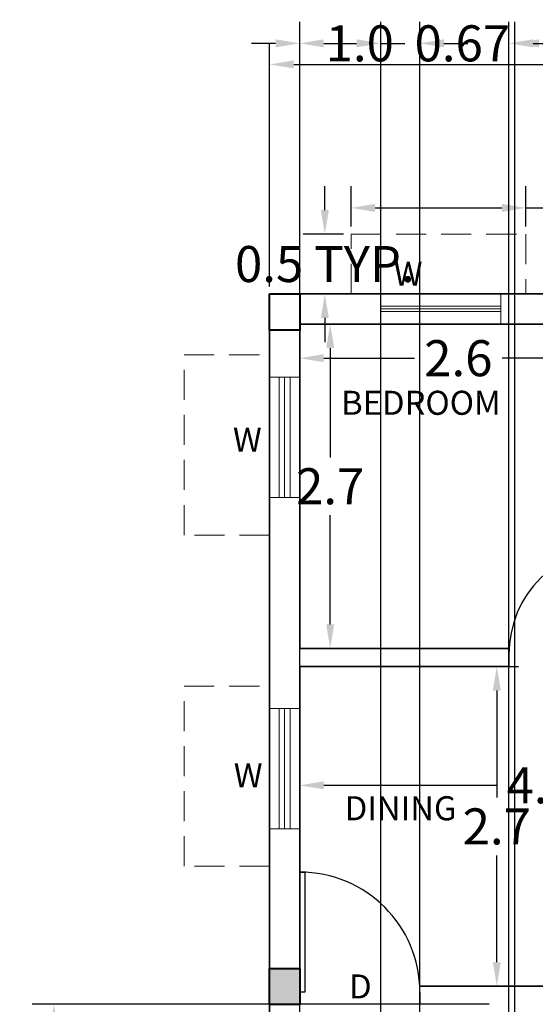
# Model space of a CAD drawing. Units: metres. Extents: x 106.5 to 121.4, y 89.1 to 111.8.
# Tile 4 of 5: x 108.1 to 112.4, y 103.6 to 111.8. Entities that reach past the tile are written whole.
import ezdxf

# ---------------------------------------------------------------- set-up
doc = ezdxf.new("R2010")
doc.units = ezdxf.units.M
doc.header["$MEASUREMENT"] = 0
doc.linetypes.add('HIDDEN', pattern=[0.375, 0.25, -0.125])
doc.layers.get('0').update_dxf_attribs({"color": 1})
for name, color, linetype, lineweight in [('A-ANNO-DIMS', 5, 'Continuous', 18), ('A-ANNO-TEXT', 4, 'Continuous', 18), ('A-AREA-IDEN', 4, 'Continuous', 18), ('A-COLS-PATT', 18, 'Continuous', 13), ('A-WALL', 1, 'Continuous', 35), ('COLUMN', 244, 'Continuous', 40), ('DR', 2, 'Continuous', 25), ('LNTL', 240, 'HIDDEN', 18), ('WNDW', 3, 'Continuous', 18)]:
    doc.layers.add(name, color=color, linetype=linetype, lineweight=lineweight)
doc.styles.get("Standard").update_dxf_attribs({"font": 'arial.ttf'})
doc.dimstyles.get("Standard").update_dxf_attribs({"dimtxt": 0.3, "dimasz": 0.2, "dimexe": 0.18, "dimexo": 0.0625, "dimgap": 0.09, "dimtad": 0, "dimtih": 1, "dimtoh": 1, "dimdec": 1, "dimzin": 0, "dimdsep": 46, "dimtxsty": 'Standard', "dimcen": 0.09, "dimadec": 0, "dimazin": 0, "dimtfac": 1, "dimtdec": 1, "dimtofl": 0, "dimtmove": 0, "dimatfit": 3, "dimfxl": 1, "dimtolj": 1, "dimtzin": 0, "dimarcsym": 0})

# ---------------------------------------------------------------- blocks, each defined once
blk = doc.blocks.new('*U2')
for p, q in [((0, 0), (0, -100)), ((-900, 0), (-900, -100))]:
    blk.add_line(p, q)
blk.add_lwpolyline([(0, 0), (0, 900), (-43.75, 900), (-43.75, 0)], close=True)
blk.add_arc((0, 0), 900, 90, 180)
blk = doc.blocks.new('*U5')
for p, q in [((0, 0), (0, -100)), ((1000, 0), (1000, -100))]:
    blk.add_line(p, q)
blk.add_lwpolyline([(0, 0), (0, 1000), (43.75, 1000), (43.75, 0)], close=True)
blk.add_arc((0, 0), 1000, 0, 90)
blk = doc.blocks.new('*D7')
at = {"layer": 'A-ANNO-DIMS', "color": 0, "lineweight": -2, "ltscale": 0.5, "transparency": 16777216}
for p, q in [((110.2029, 109.5663), (110.2029, 111.5934)), ((117.7829, 109.5663), (117.7829, 111.5934)), ((110.4029, 111.4134), (113.6312, 111.4134)), ((117.5829, 111.4134), (114.3547, 111.4134))]:
    blk.add_line(p, q, dxfattribs=at)
at = {"layer": 'A-ANNO-DIMS', "color": 0, "lineweight": -3, "ltscale": 0.5, "transparency": 16777216}
for points in [[(110.4029, 111.4467), (110.4029, 111.3801), (110.2029, 111.4134)], [(117.5829, 111.4467), (117.5829, 111.3801), (117.7829, 111.4134)]]:
    blk.add_solid(points, dxfattribs=at)
at = {"layer": 'Defpoints', "color": 0, "lineweight": -3, "ltscale": 0.5, "transparency": 16777216}
for p in [(117.7829, 111.4134), (110.2029, 109.5038), (117.7829, 109.5038)]:
    blk.add_point(p, dxfattribs=at)
at = {"layer": 'A-ANNO-DIMS', "color": 0, "ltscale": 0.5, "transparency": 16777216, "insert": (113.9929, 111.4134), "char_height": 0.3, "attachment_point": 5}
blk.add_mtext('\\A1;7.6', dxfattribs=at)
blk = doc.blocks.new('*D9')
at = {"layer": 'A-ANNO-DIMS', "color": 0, "lineweight": -2, "ltscale": 0.5, "transparency": 16777216}
for p, q in [((112.2429, 103.5313), (112.2429, 102.5093)), ((117.5329, 103.5371), (117.5329, 102.5093)), ((112.4429, 102.6893), (114.5248, 102.6893)), ((117.3329, 102.6893), (115.251, 102.6893))]:
    blk.add_line(p, q, dxfattribs=at)
at = {"layer": 'A-ANNO-DIMS', "color": 0, "lineweight": -3, "ltscale": 0.5, "transparency": 16777216}
for points in [[(112.4429, 102.7226), (112.4429, 102.6559), (112.2429, 102.6893)], [(117.3329, 102.7226), (117.3329, 102.6559), (117.5329, 102.6893)]]:
    blk.add_solid(points, dxfattribs=at)
at = {"layer": 'Defpoints', "color": 0, "lineweight": -3, "ltscale": 0.5, "transparency": 16777216}
for p in [(112.2429, 103.5938), (117.5329, 103.5996), (117.5329, 102.6893)]:
    blk.add_point(p, dxfattribs=at)
at = {"layer": 'A-ANNO-DIMS', "color": 0, "ltscale": 0.5, "transparency": 16777216, "insert": (114.8879, 102.6893), "char_height": 0.3, "attachment_point": 5}
blk.add_mtext('\\A1;5.3', dxfattribs=at)
blk = doc.blocks.new('*D18')
at = {"layer": 'A-ANNO-DIMS', "color": 0, "lineweight": -2, "ltscale": 0.5, "transparency": 16777216}
for p, q in [((110.4529, 109.0319), (110.4529, 109.1494)), ((113.0929, 109.0319), (113.0929, 109.1494)), ((110.6529, 108.9694), (111.4074, 108.9694)), ((112.8929, 108.9694), (112.1385, 108.9694))]:
    blk.add_line(p, q, dxfattribs=at)
at = {"layer": 'A-ANNO-DIMS', "color": 0, "lineweight": -3, "ltscale": 0.5, "transparency": 16777216}
for points in [[(110.6529, 109.0028), (110.6529, 108.9361), (110.4529, 108.9694)], [(112.8929, 109.0028), (112.8929, 108.9361), (113.0929, 108.9694)]]:
    blk.add_solid(points, dxfattribs=at)
at = {"layer": 'Defpoints', "color": 0, "lineweight": -3, "ltscale": 0.5, "transparency": 16777216}
for p in [(110.4529, 108.9694), (113.0929, 108.9694), (113.0929, 108.9694)]:
    blk.add_point(p, dxfattribs=at)
at = {"layer": 'A-ANNO-DIMS', "color": 0, "ltscale": 0.5, "transparency": 16777216, "insert": (111.7729, 108.9694), "char_height": 0.3, "attachment_point": 5}
blk.add_mtext('\\A1;2.6', dxfattribs=at)
blk = doc.blocks.new('*D19')
at = {"layer": 'A-ANNO-DIMS', "color": 0, "lineweight": -2, "ltscale": 0.5, "transparency": 16777216}
for p, q in [((110.7692, 109.2538), (110.8867, 109.2538)), ((110.7067, 109.0538), (110.7067, 108.1444)), ((110.7067, 106.7538), (110.7067, 107.6632)), ((110.7692, 106.5538), (110.8867, 106.5538))]:
    blk.add_line(p, q, dxfattribs=at)
at = {"layer": 'A-ANNO-DIMS', "color": 0, "lineweight": -3, "ltscale": 0.5, "transparency": 16777216}
for points in [[(110.6734, 109.0538), (110.7401, 109.0538), (110.7067, 109.2538)], [(110.6734, 106.7538), (110.7401, 106.7538), (110.7067, 106.5538)]]:
    blk.add_solid(points, dxfattribs=at)
at = {"layer": 'Defpoints', "color": 0, "lineweight": -3, "ltscale": 0.5, "transparency": 16777216}
for p in [(110.7067, 109.2538), (110.7067, 106.5538), (110.7067, 106.5538)]:
    blk.add_point(p, dxfattribs=at)
at = {"layer": 'A-ANNO-DIMS', "color": 0, "ltscale": 0.5, "transparency": 16777216, "insert": (110.7067, 107.9038), "char_height": 0.3, "attachment_point": 5}
blk.add_mtext('\\A1;2.7', dxfattribs=at)
blk = doc.blocks.new('*D20')
at = {"layer": 'A-ANNO-DIMS', "color": 0, "lineweight": -2, "ltscale": 0.5, "transparency": 16777216}
for p, q in [((110.4529, 105.4011), (110.4529, 105.5958)), ((114.4629, 105.4011), (114.4629, 105.5958)), ((110.6529, 105.4158), (112.0893, 105.4158)), ((114.2629, 105.4158), (112.8265, 105.4158))]:
    blk.add_line(p, q, dxfattribs=at)
at = {"layer": 'A-ANNO-DIMS', "color": 0, "lineweight": -3, "ltscale": 0.5, "transparency": 16777216}
for points in [[(110.6529, 105.4492), (110.6529, 105.3825), (110.4529, 105.4158)], [(114.2629, 105.4492), (114.2629, 105.3825), (114.4629, 105.4158)]]:
    blk.add_solid(points, dxfattribs=at)
at = {"layer": 'Defpoints', "color": 0, "lineweight": -3, "ltscale": 0.5, "transparency": 16777216}
for p in [(110.4529, 105.4158), (110.4529, 105.3386), (114.4629, 105.3386)]:
    blk.add_point(p, dxfattribs=at)
at = {"layer": 'A-ANNO-DIMS', "color": 0, "ltscale": 0.5, "transparency": 16777216, "insert": (112.4579, 105.4158), "char_height": 0.3, "attachment_point": 5}
blk.add_mtext('\\A1;4.0', dxfattribs=at)
blk = doc.blocks.new('*D21')
at = {"layer": 'A-ANNO-DIMS', "color": 0, "lineweight": -2, "ltscale": 0.5, "transparency": 16777216}
for p, q in [((111.8369, 106.4038), (112.2729, 106.4038)), ((112.0929, 106.2038), (112.0929, 105.3144)), ((112.0929, 103.9438), (112.0929, 104.8332)), ((111.8369, 103.7438), (112.2729, 103.7438))]:
    blk.add_line(p, q, dxfattribs=at)
at = {"layer": 'A-ANNO-DIMS', "color": 0, "lineweight": -3, "ltscale": 0.5, "transparency": 16777216}
for points in [[(112.0596, 106.2038), (112.1263, 106.2038), (112.0929, 106.4038)], [(112.0596, 103.9438), (112.1263, 103.9438), (112.0929, 103.7438)]]:
    blk.add_solid(points, dxfattribs=at)
at = {"layer": 'Defpoints', "color": 0, "lineweight": -3, "ltscale": 0.5, "transparency": 16777216}
for p in [(111.7744, 106.4038), (111.7744, 103.7438), (112.0929, 103.7438)]:
    blk.add_point(p, dxfattribs=at)
at = {"layer": 'A-ANNO-DIMS', "color": 0, "ltscale": 0.5, "transparency": 16777216, "insert": (112.0929, 105.0738), "char_height": 0.3, "attachment_point": 5}
blk.add_mtext('\\A1;2.7', dxfattribs=at)
blk = doc.blocks.new('WIN-1000-SIDE')
for p, q in [((0.0782, 0.9998), (0.0782, -0.0002)), ((0.1249, 0.9998), (0.1249, -0.0002)), ((0.1718, -0.0002), (0.1718, 0.9998))]:
    blk.add_line(p, q)
blk.add_lwpolyline([(-0.0001, 0.9998), (0.2499, 0.9998), (0.2499, -0.0002), (-0.0001, -0.0002)], close=True)
blk = doc.blocks.new('WIN-1000-END')
for p, q in [((-0.0003, 0.1472), (0.9997, 0.1472)), ((-0.0003, 0.1248), (0.9997, 0.1248)), ((-0.0003, 0.1026), (0.9997, 0.1026))]:
    blk.add_line(p, q)
blk.add_lwpolyline([(-0.0003, 0.2498), (0.9997, 0.2498), (0.9997, -0.0002), (-0.0003, -0.0002)], close=True)
blk = doc.blocks.new('LINTEL-PROJ-1498')
for p, q in [((0.0003, -0.0001), (0.0003, 1.4981)), ((0.0003, 1.4981), (0.7109, 1.4981)), ((0.7109, -0.0001), (0.0003, -0.0001))]:
    blk.add_line(p, q)
blk = doc.blocks.new('LINTEL-PROJ-1456')
for p, q in [((0.0005, -0.0002), (0.0005, 0.4976)), ((0.0005, 0.4976), (1.4557, 0.4976)), ((1.4557, 0.4976), (1.4557, -0.0002))]:
    blk.add_line(p, q)
blk = doc.blocks.new('COL-250X300')
at = {"ltscale": 0.5}
blk.add_lwpolyline([(-0.0001, 0.2999), (0.2499, 0.2999), (0.2499, -0.0001), (-0.0001, -0.0001)], close=True, dxfattribs=at)
blk = doc.blocks.new('*D52')
at = {"layer": 'A-ANNO-DIMS', "color": 0, "lineweight": -2, "ltscale": 0.5, "transparency": 16777216}
for p, q in [((110.8805, 110.0641), (110.8805, 110.3999)), ((112.3357, 110.0641), (112.3357, 110.3999)), ((111.0805, 110.2199), (112.1357, 110.2199)), ((112.3357, 110.2199), (112.5357, 110.2199))]:
    blk.add_line(p, q, dxfattribs=at)
at = {"layer": 'A-ANNO-DIMS', "color": 0, "lineweight": -3, "ltscale": 0.5, "transparency": 16777216}
for points in [[(111.0805, 110.2532), (111.0805, 110.1865), (110.8805, 110.2199)], [(112.1357, 110.2532), (112.1357, 110.1865), (112.3357, 110.2199)]]:
    blk.add_solid(points, dxfattribs=at)
at = {"layer": 'Defpoints', "color": 0, "lineweight": -3, "ltscale": 0.5, "transparency": 16777216}
for p in [(112.3357, 110.2199), (110.8805, 110.0016), (112.3357, 110.0016)]:
    blk.add_point(p, dxfattribs=at)
at = {"layer": 'A-ANNO-DIMS', "color": 0, "ltscale": 0.5, "transparency": 16777216, "insert": (113.978, 110.2199), "char_height": 0.3, "attachment_point": 5}
blk.add_mtext('\\A1;LINT. 1.5 TYP.', dxfattribs=at)
blk = doc.blocks.new('*D53')
at = {"layer": 'A-ANNO-DIMS', "color": 0, "lineweight": -2, "ltscale": 0.5, "transparency": 16777216}
for p, q in [((110.6622, 110.2016), (110.6622, 110.4016)), ((110.818, 110.0016), (110.4822, 110.0016)), ((110.818, 109.5038), (110.4822, 109.5038)), ((110.6622, 109.3038), (110.6622, 109.1038))]:
    blk.add_line(p, q, dxfattribs=at)
at = {"layer": 'A-ANNO-DIMS', "color": 0, "lineweight": -3, "ltscale": 0.5, "transparency": 16777216}
for points in [[(110.6289, 110.2016), (110.6955, 110.2016), (110.6622, 110.0016)], [(110.6289, 109.3038), (110.6955, 109.3038), (110.6622, 109.5038)]]:
    blk.add_solid(points, dxfattribs=at)
at = {"layer": 'Defpoints', "color": 0, "lineweight": -3, "ltscale": 0.5, "transparency": 16777216}
for p in [(110.6622, 110.0016), (110.8805, 110.0016), (110.8805, 109.5038)]:
    blk.add_point(p, dxfattribs=at)
at = {"layer": 'A-ANNO-DIMS', "color": 0, "ltscale": 0.5, "transparency": 16777216, "insert": (110.6622, 109.7527), "char_height": 0.3, "attachment_point": 5}
blk.add_mtext('\\A1;0.5 TYP.', dxfattribs=at)
blk = doc.blocks.new('*D58')
at = {"layer": 'A-ANNO-DIMS', "color": 0, "lineweight": -2, "ltscale": 0.5, "transparency": 16777216}
for p, q in [((110.4529, 97.2063), (110.4529, 111.7688)), ((111.4529, 97.1762), (111.4529, 111.7688)), ((110.2529, 111.5888), (110.0529, 111.5888)), ((111.6529, 111.5888), (111.8529, 111.5888))]:
    blk.add_line(p, q, dxfattribs=at)
at = {"layer": 'A-ANNO-DIMS', "color": 0, "lineweight": -3, "ltscale": 0.5, "transparency": 16777216}
for points in [[(110.2529, 111.6221), (110.2529, 111.5555), (110.4529, 111.5888)], [(111.6529, 111.6221), (111.6529, 111.5555), (111.4529, 111.5888)]]:
    blk.add_solid(points, dxfattribs=at)
at = {"layer": 'Defpoints', "color": 0, "lineweight": -3, "ltscale": 0.5, "transparency": 16777216}
for p in [(111.4529, 111.5888), (110.4529, 97.1438), (111.4529, 97.1137)]:
    blk.add_point(p, dxfattribs=at)
at = {"layer": 'A-ANNO-DIMS', "color": 0, "ltscale": 0.5, "transparency": 16777216, "insert": (110.9529, 111.5888), "char_height": 0.3, "attachment_point": 5}
blk.add_mtext('\\A1;1.0', dxfattribs=at)
blk = doc.blocks.new('*D59')
at = {"layer": 'A-ANNO-DIMS', "color": 0, "lineweight": -2, "ltscale": 0.5, "transparency": 16777216}
for p, q in [((112.1943, 94.3463), (112.1943, 111.7688)), ((113.0929, 94.3463), (113.0929, 111.7688)), ((112.3943, 111.5888), (112.8929, 111.5888)), ((113.0929, 111.5888), (113.2929, 111.5888))]:
    blk.add_line(p, q, dxfattribs=at)
at = {"layer": 'A-ANNO-DIMS', "color": 0, "lineweight": -3, "ltscale": 0.5, "transparency": 16777216}
for points in [[(112.3943, 111.6221), (112.3943, 111.5555), (112.1943, 111.5888)], [(112.8929, 111.6221), (112.8929, 111.5555), (113.0929, 111.5888)]]:
    blk.add_solid(points, dxfattribs=at)
at = {"layer": 'Defpoints', "color": 0, "lineweight": -3, "ltscale": 0.5, "transparency": 16777216}
for p in [(113.0929, 111.5888), (112.1943, 94.2838), (113.0929, 94.2838)]:
    blk.add_point(p, dxfattribs=at)
at = {"layer": 'A-ANNO-DIMS', "color": 0, "ltscale": 0.5, "transparency": 16777216, "insert": (113.772, 111.5888), "char_height": 0.3, "attachment_point": 5}
blk.add_mtext('\\A1;0.90', dxfattribs=at)
blk = doc.blocks.new('*D63')
at = {"layer": 'A-ANNO-DIMS', "color": 0, "lineweight": -2, "ltscale": 0.5, "transparency": 16777216}
for p, q in [((110.4529, 91.6463), (110.4529, 111.7688)), ((111.1267, 91.6463), (111.1267, 111.7688)), ((110.6529, 111.5888), (110.9267, 111.5888)), ((111.1267, 111.5888), (111.3267, 111.5888))]:
    blk.add_line(p, q, dxfattribs=at)
at = {"layer": 'A-ANNO-DIMS', "color": 0, "lineweight": -3, "ltscale": 0.5, "transparency": 16777216}
for points in [[(110.6529, 111.6221), (110.6529, 111.5555), (110.4529, 111.5888)], [(110.9267, 111.6221), (110.9267, 111.5555), (111.1267, 111.5888)]]:
    blk.add_solid(points, dxfattribs=at)
at = {"layer": 'Defpoints', "color": 0, "lineweight": -3, "ltscale": 0.5, "transparency": 16777216}
for p in [(111.1267, 111.5888), (110.4529, 91.5838), (111.1267, 91.5838)]:
    blk.add_point(p, dxfattribs=at)
at = {"layer": 'A-ANNO-DIMS', "color": 0, "ltscale": 0.5, "transparency": 16777216, "insert": (111.8063, 111.5888), "char_height": 0.3, "attachment_point": 5}
blk.add_mtext('\\A1;0.67', dxfattribs=at)
blk = doc.blocks.new('*D72')
at = {"layer": 'A-ANNO-DIMS', "color": 0, "lineweight": -2, "ltscale": 0.5, "transparency": 16777216}
for p, q in [((112.2429, 98.9563), (112.2429, 111.7688)), ((113.7429, 98.9563), (113.7429, 111.7688)), ((112.4429, 111.5888), (112.6428, 111.5888)), ((113.5429, 111.5888), (113.343, 111.5888))]:
    blk.add_line(p, q, dxfattribs=at)
at = {"layer": 'A-ANNO-DIMS', "color": 0, "lineweight": -3, "ltscale": 0.5, "transparency": 16777216}
for points in [[(112.4429, 111.6221), (112.4429, 111.5555), (112.2429, 111.5888)], [(113.5429, 111.6221), (113.5429, 111.5555), (113.7429, 111.5888)]]:
    blk.add_solid(points, dxfattribs=at)
at = {"layer": 'Defpoints', "color": 0, "lineweight": -3, "ltscale": 0.5, "transparency": 16777216}
for p in [(113.7429, 111.5888), (112.2429, 98.8938), (113.7429, 98.8938)]:
    blk.add_point(p, dxfattribs=at)
at = {"layer": 'A-ANNO-DIMS', "color": 0, "ltscale": 0.5, "transparency": 16777216, "insert": (112.9929, 111.5888), "char_height": 0.3, "attachment_point": 5}
blk.add_mtext('\\A1;1.5', dxfattribs=at)
blk = doc.blocks.new('*D77')
at = {"layer": 'A-ANNO-DIMS', "color": 0, "lineweight": -2, "ltscale": 0.5, "transparency": 16777216}
for p, q in [((112.0304, 103.5938), (108.2273, 103.5938)), ((108.4073, 103.3938), (108.4073, 103.037)), ((108.4073, 102.1938), (108.4073, 102.5506)), ((112.0304, 101.9938), (108.2273, 101.9938))]:
    blk.add_line(p, q, dxfattribs=at)
at = {"layer": 'A-ANNO-DIMS', "color": 0, "lineweight": -3, "ltscale": 0.5, "transparency": 16777216}
for points in [[(108.3739, 103.3938), (108.4406, 103.3938), (108.4073, 103.5938)], [(108.3739, 102.1938), (108.4406, 102.1938), (108.4073, 101.9938)]]:
    blk.add_solid(points, dxfattribs=at)
at = {"layer": 'Defpoints', "color": 0, "lineweight": -3, "ltscale": 0.5, "transparency": 16777216}
for p in [(108.4073, 103.5938), (112.0929, 103.5938), (112.0929, 101.9938)]:
    blk.add_point(p, dxfattribs=at)
at = {"layer": 'A-ANNO-DIMS', "color": 0, "ltscale": 0.5, "transparency": 16777216, "insert": (108.4073, 102.7938), "char_height": 0.3, "attachment_point": 5}
blk.add_mtext('\\A1;1.6', dxfattribs=at)

msp = doc.modelspace()

# ---------------------------------------------------------------- hatches: boundary and pattern name
at = {"layer": 'A-COLS-PATT', "ltscale": 0.5}
h = msp.add_hatch(dxfattribs=at)
h.set_pattern_fill('CORK', color=256, scale=10)
h.set_pattern_definition([(0, (0, 0), (0, 1.25), []), (135, (0.625, -0.625), (-2.5, -2.5), [1.76777, -1.76777]), (135, (0.9375, -0.625), (-2.5, -2.5), [1.76777, -1.76777]), (135, (1.25, -0.625), (-2.5, -2.5), [1.76777, -1.76777])])
h.paths.add_polyline_path([(110.2029, 109.5038), (110.2029, 109.2038), (110.4529, 109.2038), (110.4529, 109.5038)])
h.paths.add_polyline_path([(114.6132, 109.5038), (114.3632, 109.5038), (114.3632, 109.2538), (114.4629, 109.2538), (114.4629, 109.2038), (114.6129, 109.2038), (114.6129, 109.2538)])
h.paths.add_polyline_path([(117.5321, 109.2538), (117.5329, 109.2538), (117.5329, 109.2038), (117.7821, 109.2038), (117.7821, 109.5038), (117.5321, 109.5038)])
h = msp.add_hatch(color=256, dxfattribs=at)
h.dxf.hatch_style = 1
h.paths.add_polyline_path([(110.4529, 103.8929), (110.2029, 103.8929), (110.2029, 103.5938), (110.4529, 103.5938)])
h.paths.add_polyline_path([(114.4629, 103.8938), (114.3632, 103.8938), (114.3632, 103.7438), (114.4629, 103.7438)])
h.paths.add_polyline_path([(114.6129, 103.8938), (114.4629, 103.8938), (114.4629, 103.7438), (114.6129, 103.7438)])
h.paths.add_polyline_path([(114.6132, 103.7438), (114.4629, 103.7438), (114.3632, 103.7438), (114.3632, 103.5938), (114.6132, 103.5938)])
h.paths.add_polyline_path([(117.7829, 103.8996), (117.5329, 103.8996), (117.5329, 103.5996), (117.7829, 103.5996)])
h.paths.add_polyline_path([(117.7829, 98.888), (117.5329, 98.888), (117.5329, 98.588), (117.7829, 98.588)])
h.paths.add_polyline_path([(110.4529, 98.8938), (110.2029, 98.8938), (110.2029, 98.5947), (110.4529, 98.5947)])
h.paths.add_polyline_path([(114.6132, 98.8938), (114.3132, 98.8938), (114.3132, 98.7438), (114.4632, 98.7438), (114.6132, 98.7438)])
h.paths.add_polyline_path([(110.4529, 91.6338), (110.2029, 91.6338), (110.2029, 91.3338), (110.4529, 91.3338)])
h.paths.add_polyline_path([(114.6132, 91.5838), (114.6129, 91.5838), (114.6129, 91.6338), (114.4629, 91.6338), (114.4629, 91.5838), (114.3632, 91.5838), (114.3632, 91.3338), (114.6132, 91.3338)])
h.paths.add_polyline_path([(117.7821, 91.6338), (117.5329, 91.6338), (117.5329, 91.5838), (117.5321, 91.3338), (117.7821, 91.3338)])

# ---------------------------------------------------------------- linework, layer by layer
at = {"layer": 'A-WALL'}
for p, q in [((117.7829, 109.5038), (110.2029, 109.5038)), ((110.2029, 109.5038), (110.2029, 101.3638)), ((110.4529, 109.2538), (110.4529, 106.5538)), ((113.0929, 109.2538), (110.4529, 109.2538)), ((112.1943, 106.5538), (110.4529, 106.5538)), ((112.1929, 106.4038), (110.4529, 106.4038)), ((110.4529, 106.4038), (110.4529, 103.7438)), ((114.6129, 103.7438), (111.4517, 103.7438))]:
    msp.add_line(p, q, dxfattribs=at)
at = {"layer": 'COLUMN', "ltscale": 0.5}
msp.add_lwpolyline([(110.2029, 109.5038), (110.4529, 109.5038), (110.4529, 109.2038), (110.2029, 109.2038)], close=True, dxfattribs=at)
at = {"layer": 'WNDW'}
for p, q in [((110.2812, 106.0547), (110.2812, 105.0547)), ((110.3279, 106.0547), (110.3279, 105.0547)), ((110.3748, 105.0547), (110.3748, 106.0547))]:
    msp.add_line(p, q, dxfattribs=at)
msp.add_lwpolyline([(110.2029, 106.0547), (110.4529, 106.0547), (110.4529, 105.0547), (110.2029, 105.0547)], close=True, dxfattribs=at)

# ---------------------------------------------------------------- block references
at = {"layer": 'COLUMN'}
msp.add_blockref('COL-250X300', (110.203, 103.593), dxfattribs=at)
at = {"layer": 'DR', "xscale": 0.001, "yscale": 0.001, "zscale": 0.001}
for name, p in [('*U2', (113.0929, 106.5038)), ('*U5', (110.4529, 103.6938))]:
    msp.add_blockref(name, p, dxfattribs=at)
at = {"layer": 'LNTL'}
for name, p in [('LINTEL-PROJ-1456', (110.88, 109.504)), ('LINTEL-PROJ-1498', (109.492, 107.498)), ('LINTEL-PROJ-1498', (109.492, 104.7419))]:
    msp.add_blockref(name, p, dxfattribs=at)
at = {"layer": 'WNDW'}
for name, p in [('WIN-1000-END', (111.127, 109.254)), ('WIN-1000-SIDE', (110.203, 107.811))]:
    msp.add_blockref(name, p, dxfattribs=at)

# ---------------------------------------------------------------- texts
at = {"layer": 'A-ANNO-TEXT', "ltscale": 0.5, "char_height": 0.2, "attachment_point": 1}
for s, width, insert in [('W', 0.390771, (111.2359, 109.7716)), ('W', 0.390771, (109.8975, 108.3914)), ('W', 0.390771, (109.9045, 105.5988)), ('D', 0.320447, (110.8641, 103.8424))]:
    msp.add_mtext_dynamic_manual_height_columns(s, width=width, gutter_width=1, heights=[0], dxfattribs=dict(at, insert=insert))
at = {"layer": 'A-AREA-IDEN', "ltscale": 0.5, "char_height": 0.2, "attachment_point": 1}
for s, insert in [('BEDROOM', (110.7979, 108.6983)), ('DINING', (110.8277, 105.3249))]:
    msp.add_mtext_dynamic_manual_height_columns(s, width=0.914899, gutter_width=1, heights=[0], dxfattribs=dict(at, insert=insert))

# ---------------------------------------------------------------- dimensions: what is measured, and where the dimension line sits
at = {"layer": 'A-ANNO-DIMS', "ltscale": 0.5}
for base, p1, p2, override, picture, middle in [((111.4529, 111.5888), (110.4529, 97.1438), (111.4529, 97.1137), {"dimdec": 1, "dimlfac": 1, "dimrnd": 0, "dimzin": 0, "dimdsep": 46, "dimlunit": 2}, '*D58', (110.9529, 111.5888)), ((111.1267, 111.5888), (110.4529, 91.5838), (111.1267, 91.5838), {"dimdec": 2, "dimlfac": 1, "dimrnd": 0, "dimzin": 0, "dimdsep": 46, "dimlunit": 2}, '*D63', (111.8063, 111.5888)), ((113.0929, 111.5888), (112.1943, 94.2838), (113.0929, 94.2838), {"dimdec": 2, "dimlfac": 1, "dimrnd": 0, "dimzin": 0, "dimdsep": 46, "dimlunit": 2}, '*D59', (113.772, 111.5888)), ((113.7429, 111.5888), (112.2429, 98.8938), (113.7429, 98.8938), {"dimdec": 1, "dimlfac": 1, "dimrnd": 0, "dimzin": 0, "dimdsep": 46, "dimlunit": 2}, '*D72', (112.9929, 111.5888)), ((117.7829, 111.4134), (110.2029, 109.5038), (117.7829, 109.5038), {"dimclrd": 0, "dimclre": 0, "dimclrt": 0}, '*D7', (113.9929, 111.4134)), ((113.0929, 108.9694), (110.4529, 108.9694), (113.0929, 108.9694), {"dimclrd": 0, "dimclre": 0, "dimclrt": 0}, '*D18', (111.7729, 108.9694)), ((110.4529, 105.4158), (114.4629, 105.3386), (110.4529, 105.3386), {"dimclrd": 0, "dimclre": 0, "dimclrt": 0}, '*D20', (112.4579, 105.4158)), ((117.5329, 102.6893), (112.2429, 103.5938), (117.5329, 103.5996), {"dimclrd": 0, "dimclre": 0, "dimclrt": 0}, '*D9', (114.8879, 102.6893))]:
    dim = msp.add_linear_dim(base=base, p1=p1, p2=p2, dimstyle='Standard', override=override, dxfattribs=at)
    dim.commit()
    dim.dimension.update_dxf_attribs({"geometry": picture, "text_midpoint": middle})
dim = msp.add_linear_dim(base=(112.3357, 110.2199), p1=(110.8805, 110.0016), p2=(112.3357, 110.0016), text='LINT. <> TYP.', dimstyle='Standard', override={"dimdec": 1, "dimlfac": 1, "dimrnd": 0, "dimzin": 0, "dimdsep": 46, "dimlunit": 2}, dxfattribs=at)
dim.commit()
dim.dimension.update_dxf_attribs({"geometry": '*D52', "text_midpoint": (113.978, 110.2199)})
dim = msp.add_linear_dim(base=(110.6622, 110.0016), p1=(110.8805, 109.5038), p2=(110.8805, 110.0016), angle=90, text='<> TYP.', dimstyle='Standard', override={"dimdec": 1, "dimlfac": 1, "dimrnd": 0, "dimzin": 0, "dimdsep": 46, "dimlunit": 2}, dxfattribs=at)
dim.commit()
dim.dimension.update_dxf_attribs({"geometry": '*D53', "text_midpoint": (110.6622, 109.7527)})
for base, p1, p2, override, picture, middle in [((110.7067, 106.5538), (110.7067, 109.2538), (110.7067, 106.5538), {"dimclrd": 0, "dimclre": 0, "dimclrt": 0}, '*D19', (110.7067, 107.9038)), ((112.0929, 103.7438), (111.7744, 106.4038), (111.7744, 103.7438), {"dimclrd": 0, "dimclre": 0, "dimclrt": 0}, '*D21', (112.0929, 105.0738)), ((108.4073, 103.5938), (112.0929, 101.9938), (112.0929, 103.5938), {"dimdec": 1, "dimlfac": 1, "dimrnd": 0, "dimzin": 0, "dimdsep": 46, "dimlunit": 2}, '*D77', (108.4073, 102.7938))]:
    dim = msp.add_linear_dim(base=base, p1=p1, p2=p2, angle=90, dimstyle='Standard', override=override, dxfattribs=at)
    dim.commit()
    dim.dimension.update_dxf_attribs({"geometry": picture, "text_midpoint": middle})

doc.saveas('drawing.dxf')
